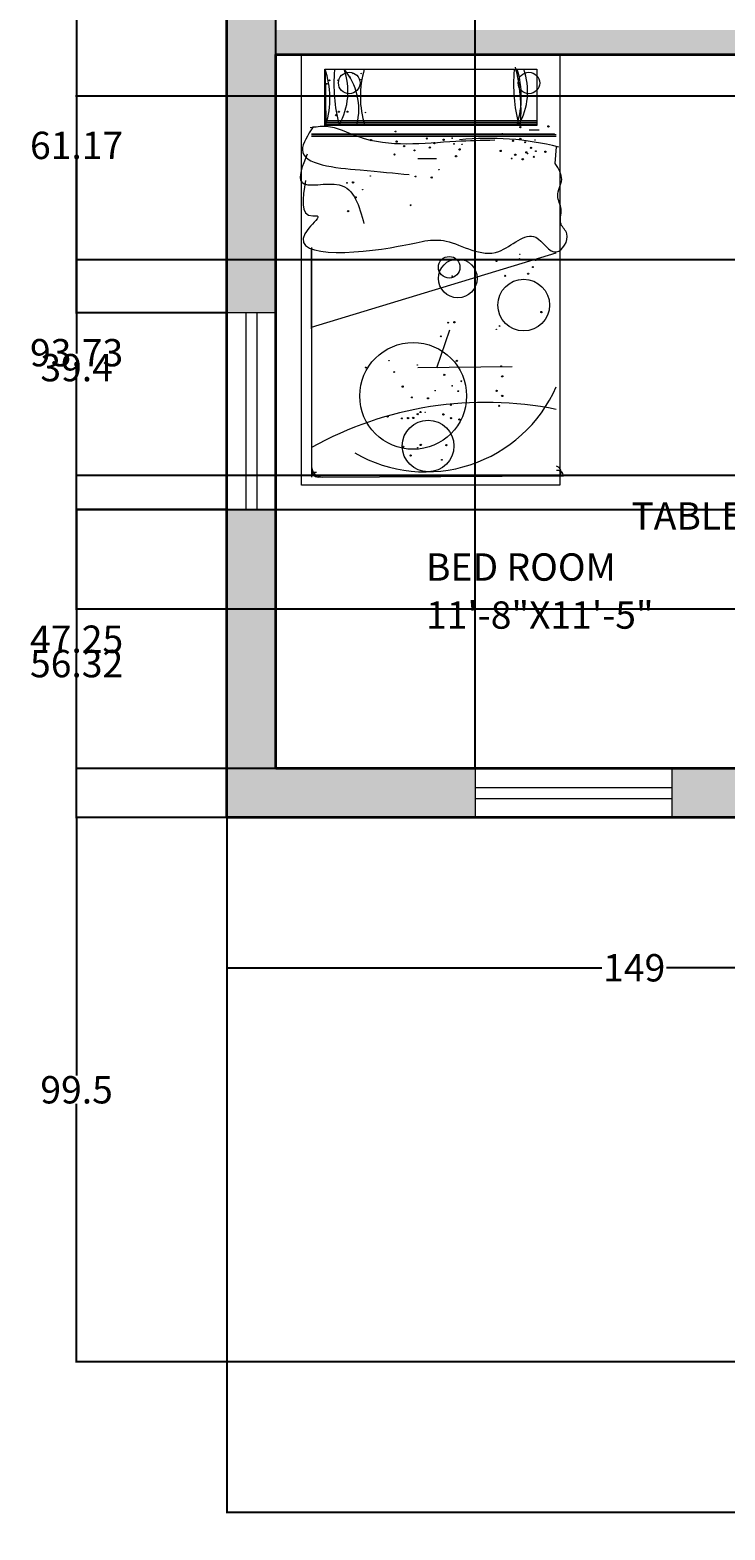
# Model space of a CAD drawing. Units: inches. Extents: x 2807 to 3326, y 2005 to 2580.
# Tile 1 of 12: x 2809 to 2936, y 2005 to 2280. Entities that reach past the tile are written whole.
import ezdxf

# ---------------------------------------------------------------- set-up
doc = ezdxf.new("R2010")
doc.units = ezdxf.units.IN
doc.header["$LTSCALE"] = 0.4
for name, color, linetype, lineweight in [('A-ANNO-DIMS', 2, 'Continuous', 18), ('A-AREA-IDEN', 5, 'Continuous', 18), ('A-WALL-PATT', 231, 'Continuous', 13), ('Furniture', 7, 'Continuous', 15), ('WALL', 233, 'Continuous', 35), ('WINDOWS', 132, 'Continuous', 18)]:
    doc.layers.add(name, color=color, linetype=linetype, lineweight=lineweight)
doc.styles.get("Standard").update_dxf_attribs({"font": 'txt', "height": 5})
doc.dimstyles.get("Standard").update_dxf_attribs({"dimtxt": 0.18, "dimasz": 0.18, "dimexe": 0.18, "dimexo": 0.0625, "dimgap": 0.09, "dimtad": 0, "dimtih": 1, "dimtoh": 1, "dimdec": 4, "dimzin": 0, "dimdsep": 46, "dimtxsty": 'Standard', "dimcen": 0.09, "dimadec": 0, "dimazin": 0, "dimtfac": 1, "dimtdec": 4, "dimtofl": 0, "dimtmove": 0, "dimatfit": 3, "dimfxl": 1, "dimtolj": 1, "dimtzin": 0, "dimarcsym": 0})

# ---------------------------------------------------------------- blocks, each defined once
blk = doc.blocks.new('WIN-36')
at = {"ltscale": 0.4}
for p, q in [((0, 36), (0, 0)), ((9, 36), (0, 36)), ((3.5, 36), (3.5, 0)), ((5.5, 36), (5.5, 0)), ((9, 0), (9, 36)), ((0, 0), (9, 0))]:
    blk.add_line(p, q, dxfattribs=at)
blk = doc.blocks.new('BED-SINGLE')
for p, q in [((-24.2, -78.74), (-24.2, 0)), ((23.05, 0), (-24.2, 0)), ((23.05, 0), (23.05, -78.74)), ((-19.91, -2.64), (18.85, -2.64)), ((-19.91, -12.97), (-19.91, -2.64)), ((-19.86, -2.65), (-19.71, -12.79)), ((18.85, -2.64), (18.85, -12.97)), ((18.85, -12.97), (-19.91, -12.97)), ((-19.71, -12.07), (18.88, -12.07)), ((-19.71, -12.36), (18.88, -12.36)), ((-19.71, -12.66), (18.88, -12.66)), ((-19.71, -12.79), (18.88, -12.79)), ((-22.36, -14.62), (22.4, -14.6)), ((-22.36, -14.92), (22.4, -14.9)), ((-22.34, -14.47), (22.1, -14.45)), ((19.29, -13.84), (17.45, -13.84)), ((0.5, -19.06), (-2.92, -19.06)), ((22.21, -19.89), (22.42, -16.84)), ((-22.34, -35.25), (-22.34, -77.26)), ((-22.34, -35.25), (-22.34, -75.28)), ((-22.34, -50.11), (-22.34, -35.53)), ((-22.36, -49.81), (22.4, -36.21)), ((2.87, -50.36), (0.49, -57.3)), ((14.32, -57.07), (-2.92, -57.29)), ((-22.21, -76.32), (-21.42, -76.32)), ((23.05, -78.74), (-24.2, -78.74)), ((-21.16, -77.25), (23.72, -77.02))]:
    blk.add_line(p, q)
for centre, radius in [((-19.54, -5.33), 0.0787), ((-19.07, -4.7), 0.0787), ((-17.49, -4.7), 0.0787), ((-15.45, -5.18), 1.97), ((-15.29, -4.08), 0.0394), ((-14.82, -3.45), 0.0394), ((-13.24, -3.45), 0.0394), ((-13.24, -4.55), 0.0394), ((17.4, -5.19), 1.97), ((-17.82, -11.05), 0.118), ((-17.35, -10.43), 0.118), ((-15.77, -10.43), 0.118), ((-12.46, -10.58), 0.0394), ((15.84, -13.26), 0.118), ((20.96, -13.12), 0.118), ((-11.46, -15.62), 0.118), ((-6.97, -14.05), 0.0787), ((-6.78, -15.9), 0.118), ((-1.26, -15.34), 0.118), ((0.11, -16.17), 0.118), ((1.8, -15.56), 0.118), ((3.7, -16.3), 0.0787), ((5.19, -16.39), 0.0394), ((12.55, -14.52), 0.118), ((14.47, -15.76), 0.118), ((15.82, -15.39), 0.118), ((16.73, -16.02), 0.0787), ((17.27, -14.65), 0.0394), ((18.52, -15.61), 0.0394), ((-7.18, -18.26), 0.118), ((-5.4, -16.72), 0.118), ((-3.52, -17.51), 0.0787), ((-0.71, -17), 0.118), ((4.08, -18.58), 0.118), ((4.72, -17.32), 0.118), ((12.24, -17.6), 0.118), ((14.25, -19), 0.0787), ((14.9, -18.3), 0.118), ((16.28, -19.13), 0.118), ((16.93, -17.87), 0.118), ((17.15, -18.11), 0.0394), ((17.76, -17.04), 0.118), ((18.3, -18.69), 0.118), ((18.66, -17.64), 0.0787), ((20.41, -17.75), 0.118), ((0.94, -21.04), 0.0394), ((-15.86, -23.43), 0.0787), ((-14.74, -23.37), 0.118), ((-12.98, -24.68), 0.0394), ((-11.61, -22.18), 0.0394), ((-3.31, -22.29), 0.0787), ((-0.37, -22.46), 0.118), ((-14.28, -26.11), 0.118), ((-15.65, -28.61), 0.118), ((-4.22, -27.54), 0.0787), ((2.83, -38.87), 1.97), ((4.4, -40.91), 3.54), ((4.64, -37.58), 0.0394), ((11.49, -37.77), 0.0787), ((15.68, -37.38), 0.0787), ((15.74, -36.51), 0.0394), ((18.63, -37.54), 0.118), ((16.45, -45.79), 4.72), ((13.06, -40.44), 0.118), ((17.26, -40.05), 0.118), ((18.11, -38.84), 0.0787), ((2.65, -49), 0.0787), ((3.77, -48.94), 0.118), ((19.68, -47.06), 0.118), ((1.28, -51.5), 0.0787), ((11.44, -50.24), 0.0394), ((12.05, -49.61), 0.0787), ((-3.76, -62.4), 9.76), ((-12.43, -57.2), 0.0787), ((-8.18, -55.94), 0.0394), ((-3, -56.76), 0.0394), ((4.23, -56), 0.118), ((12.32, -56.97), 0.0787), ((-7.25, -58.02), 0.0787), ((1.92, -58.54), 0.118), ((5.04, -59.72), 0.0787), ((12.52, -58.82), 0.118), ((-5.68, -60.69), 0.118), ((-3.99, -62.67), 0.0787), ((-1.05, -62.84), 0.118), ((0.26, -61.41), 0.0394), ((4.48, -61.53), 0.0787), ((11.5, -61.47), 0.118), ((12.52, -62.39), 0.118), ((-2.92, -65.73), 0.118), ((-2.42, -65.34), 0.118), ((-1.57, -65.38), 0.0394), ((1.77, -65.78), 0.118), ((3.11, -64.04), 0.0787), ((11.96, -64.21), 0.118), ((-8.43, -66.14), 0.118), ((-5.82, -66.51), 0.0787), ((-1.03, -71.55), 4.72), ((-4.7, -66.45), 0.118), ((-3.75, -66.42), 0.118), ((3.15, -66.47), 0.118), ((4.68, -66.71), 0.118), ((-2.37, -71.35), 0.118), ((2.32, -71.4), 0.118), ((-5.61, -71.69), 0.118), ((-4.24, -73.29), 0.118), ((-2.94, -71.86), 0.0394), ((1.48, -74.08), 0.0787)]:
    blk.add_circle(centre, radius)
for centre, radius, start, end in [((-35.51, -7.95), 16.53, 343.0006, 18.6759), ((-27.69, -6.75), 12.01, 329.8072, 19.9256), ((-25.06, -10.01), 11.36, 345.8396, 40.337), ((4.43, -7.67), 17.85, 163.6634, 197.1743), ((-14.89, -10.2), 30.85, 355.6161, 14.8863), ((-1.49, -7.71), 17.5, 343.1329, 16.7593), ((5.16, -6.76), 12.01, 329.8072, 19.9256), ((10.58, -5.48), 28.83, 174.7074, 194.6885), ((43.43, -5.5), 28.83, 174.7074, 194.6885), ((10.02, -67.77), 52.46, 75.8437, 95.7821), ((-1.46, -50.2), 26.08, 240.1506, 336.1931), ((9.49, -129.11), 65.53, 78.633, 119.0775), ((-20.37, -75.28), 1.97, 180, 270), ((-21.16, -76.07), 1.18, 180, 270), ((22.26, -76.26), 1.02, 311.9337, 80.5378), ((22.61, -77.16), 1.13, 7.0311, 99.2977)]:
    blk.add_arc(centre, radius, start, end)
for points, knots in [([(-22, -13.16), (-23.02, -14.71), (-26.47, -19.94), (-13.14, -21.11), (-7.15, -21.67), (-4.47, -21.92)], [0, 0, 0, 0, 4.712342, 15.867179, 24.91455, 24.91455, 24.91455, 24.91455]), ([(11.17, -15.66), (8.81, -15.7), (0.54, -15.87), (-10.21, -17.37), (-18.53, -12.79), (-21.61, -13.25), (-22.61, -13.4)], [0, 0, 0, 0, 7.121262, 24.909491, 31.123221, 34.101394, 34.101394, 34.101394, 34.101394]), ([(-23.16, -18.18), (-24, -20.34), (-25.96, -25.33), (-15.15, -21.84), (-13.61, -27.69), (-12.77, -30.9)], [0, 0, 0, 0, 5.247261, 12.129135, 20.530793, 20.530793, 20.530793, 20.530793]), ([(-23.42, -23.01), (-23.98, -26.23), (-24.61, -29.87), (-20.32, -29.28), (-30.03, -37.77), (-6.68, -35.83), (2.09, -32.61), (11.16, -38.92), (18.11, -30.55), (22.1, -38.17), (25.33, -33.01), (22.67, -30.96), (23.73, -28.27), (22.1, -25.67), (24.04, -22.75), (22.83, -20.86), (22.21, -19.89)], [0, 0, 0, 0, 6.608381, 7.436978, 10.160479, 26.82811, 35.651646, 45.441607, 52.697614, 57.347481, 61.162366, 63.231685, 65.951856, 68.505046, 71.545852, 74.730692, 74.730692, 74.730692, 74.730692])]:
    blk.add_open_spline(points, degree=3, knots=knots)
for p in [(3.38, -15.28), (3.38, -40.49), (3.38, -60.57)]:
    blk.add_point(p)
blk = doc.blocks.new('*D29')
at = {"layer": 'A-ANNO-DIMS', "color": 0, "lineweight": -2, "ltscale": 0.4, "transparency": 16777216}
for p, q in [((2959.79, 2230.64), (2947.71, 2230.64)), ((2947.89, 2230.46), (2947.89, 2193.32)), ((2947.89, 2151.01), (2947.89, 2188.14)), ((2959.79, 2150.83), (2947.71, 2150.83))]:
    blk.add_line(p, q, dxfattribs=at)
at = {"layer": 'A-ANNO-DIMS', "color": 0, "ltscale": 0.4, "transparency": 16777216}
for points in [[(2947.86, 2230.46), (2947.92, 2230.46), (2947.89, 2230.64)], [(2947.86, 2151.01), (2947.92, 2151.01), (2947.89, 2150.83)]]:
    blk.add_solid(points, dxfattribs=at)
at = {"layer": 'Defpoints', "color": 0, "ltscale": 0.4, "transparency": 16777216}
for p in [(2947.89, 2230.64), (2959.86, 2230.64), (2959.86, 2150.83)]:
    blk.add_point(p, dxfattribs=at)
at = {"layer": 'A-ANNO-DIMS', "color": 0, "ltscale": 0.4, "transparency": 16777216, "insert": (2947.89, 2190.73), "char_height": 5, "attachment_point": 5}
blk.add_mtext('\\A1;TABLE SET 80 TYP.', dxfattribs=at)
blk = doc.blocks.new('*D31')
at = {"layer": 'A-ANNO-DIMS', "color": 0, "lineweight": -2, "ltscale": 0.4, "transparency": 16777216}
for p, q in [((2844.57, 2135.51), (2844.57, 2008.45)), ((3288.57, 2135.51), (3288.57, 2008.45)), ((2844.75, 2008.63), (3059.93, 2008.63)), ((3288.39, 2008.63), (3073.2, 2008.63))]:
    blk.add_line(p, q, dxfattribs=at)
at = {"layer": 'A-ANNO-DIMS', "color": 0, "ltscale": 0.4, "transparency": 16777216}
for points in [[(2844.75, 2008.66), (2844.75, 2008.6), (2844.57, 2008.63)], [(3288.39, 2008.66), (3288.39, 2008.6), (3288.57, 2008.63)]]:
    blk.add_solid(points, dxfattribs=at)
at = {"layer": 'Defpoints', "color": 0, "ltscale": 0.4, "transparency": 16777216}
for p in [(2844.57, 2135.58), (3288.57, 2135.58), (3288.57, 2008.63)]:
    blk.add_point(p, dxfattribs=at)
at = {"layer": 'A-ANNO-DIMS', "color": 0, "ltscale": 0.4, "transparency": 16777216, "insert": (3066.57, 2008.63), "char_height": 5, "attachment_point": 5}
blk.add_mtext('\\A1;444', dxfattribs=at)
blk = doc.blocks.new('*D33')
at = {"layer": 'A-ANNO-DIMS', "color": 0, "lineweight": -2, "ltscale": 0.4, "transparency": 16777216}
for p, q in [((2844.504691, 2135.576496), (2816.937191, 2135.576496)), ((2817.117191, 2135.396496), (2817.117191, 2088.416496)), ((2817.117191, 2036.256496), (2817.117191, 2083.236496)), ((2984.504691, 2036.076496), (2816.937191, 2036.076496))]:
    blk.add_line(p, q, dxfattribs=at)
at = {"layer": 'A-ANNO-DIMS', "color": 0, "ltscale": 0.4, "transparency": 16777216}
for points in [[(2817.087191, 2135.396496), (2817.147191, 2135.396496), (2817.117191, 2135.576496)], [(2817.087191, 2036.256496), (2817.147191, 2036.256496), (2817.117191, 2036.076496)]]:
    blk.add_solid(points, dxfattribs=at)
at = {"layer": 'Defpoints', "color": 0, "ltscale": 0.4, "transparency": 16777216}
for p in [(2817.117191, 2135.576496), (2844.567191, 2135.576496), (2984.567191, 2036.076496)]:
    blk.add_point(p, dxfattribs=at)
at = {"layer": 'A-ANNO-DIMS', "color": 0, "ltscale": 0.4, "transparency": 16777216, "insert": (2817.117191, 2085.826496), "char_height": 5, "attachment_point": 5}
blk.add_mtext('\\A1;99.5', dxfattribs=at)
blk = doc.blocks.new('*D35')
at = {"layer": 'A-ANNO-DIMS', "color": 0, "lineweight": -2, "ltscale": 0.4, "transparency": 16777216}
for p, q in [((2844.57, 2135.51), (2844.57, 2107.95)), ((2993.57, 2135.51), (2993.57, 2107.95)), ((2844.75, 2108.13), (2913.14, 2108.13)), ((2993.39, 2108.13), (2924.99, 2108.13))]:
    blk.add_line(p, q, dxfattribs=at)
at = {"layer": 'A-ANNO-DIMS', "color": 0, "ltscale": 0.4, "transparency": 16777216}
for points in [[(2844.75, 2108.16), (2844.75, 2108.1), (2844.57, 2108.13)], [(2993.39, 2108.16), (2993.39, 2108.1), (2993.57, 2108.13)]]:
    blk.add_solid(points, dxfattribs=at)
at = {"layer": 'Defpoints', "color": 0, "ltscale": 0.4, "transparency": 16777216}
for p in [(2844.57, 2135.58), (2993.57, 2135.58), (2844.57, 2108.13)]:
    blk.add_point(p, dxfattribs=at)
at = {"layer": 'A-ANNO-DIMS', "color": 0, "ltscale": 0.4, "transparency": 16777216, "insert": (2919.07, 2108.13), "char_height": 5, "attachment_point": 5}
blk.add_mtext('\\A1;149', dxfattribs=at)
blk = doc.blocks.new('*D37')
at = {"layer": 'A-ANNO-DIMS', "color": 0, "lineweight": -2, "ltscale": 0.4, "transparency": 16777216}
for p, q in [((2853.567191, 2144.638996), (2853.567191, 2577.206496)), ((2853.747191, 2577.026496), (2859.189306, 2577.026496)), ((2889.811421, 2577.026496), (2884.369306, 2577.026496)), ((2889.991421, 2144.638996), (2889.991421, 2577.206496))]:
    blk.add_line(p, q, dxfattribs=at)
at = {"layer": 'A-ANNO-DIMS', "color": 0, "ltscale": 0.4, "transparency": 16777216}
for points in [[(2853.747191, 2577.056496), (2853.747191, 2576.996496), (2853.567191, 2577.026496)], [(2889.811421, 2577.056496), (2889.811421, 2576.996496), (2889.991421, 2577.026496)]]:
    blk.add_solid(points, dxfattribs=at)
at = {"layer": 'Defpoints', "color": 0, "ltscale": 0.4, "transparency": 16777216}
for p in [(2889.991421, 2577.026496), (2853.567191, 2144.576496), (2889.991421, 2144.576496)]:
    blk.add_point(p, dxfattribs=at)
at = {"layer": 'A-ANNO-DIMS', "color": 0, "ltscale": 0.4, "transparency": 16777216, "insert": (2871.779306, 2577.026496), "char_height": 5, "attachment_point": 5}
blk.add_mtext('\\A1;36.424', dxfattribs=at)
blk = doc.blocks.new('*D41')
at = {"layer": 'A-ANNO-DIMS', "color": 0, "lineweight": -2, "ltscale": 0.4, "transparency": 16777216}
for p, q in [((2844.5, 2191.9), (2816.94, 2191.9)), ((2817.12, 2191.72), (2817.12, 2166.33)), ((2817.12, 2135.76), (2817.12, 2161.15)), ((2844.5, 2135.58), (2816.94, 2135.58))]:
    blk.add_line(p, q, dxfattribs=at)
at = {"layer": 'A-ANNO-DIMS', "color": 0, "ltscale": 0.4, "transparency": 16777216}
for points in [[(2817.09, 2191.72), (2817.15, 2191.72), (2817.12, 2191.9)], [(2817.09, 2135.76), (2817.15, 2135.76), (2817.12, 2135.58)]]:
    blk.add_solid(points, dxfattribs=at)
at = {"layer": 'Defpoints', "color": 0, "ltscale": 0.4, "transparency": 16777216}
for p in [(2817.12, 2191.9), (2844.57, 2191.9), (2844.57, 2135.58)]:
    blk.add_point(p, dxfattribs=at)
at = {"layer": 'A-ANNO-DIMS', "color": 0, "ltscale": 0.4, "transparency": 16777216, "insert": (2817.12, 2163.74), "char_height": 5, "attachment_point": 5}
blk.add_mtext('\\A1;56.32', dxfattribs=at)
blk = doc.blocks.new('*D42')
at = {"layer": 'A-ANNO-DIMS', "color": 0, "lineweight": -2, "ltscale": 0.4, "transparency": 16777216}
for p, q in [((2844.504691, 2289.066335), (2816.937191, 2289.066335)), ((2817.117191, 2288.886335), (2817.117191, 2261.071202)), ((2817.117191, 2228.076069), (2817.117191, 2255.891202)), ((2844.504691, 2227.896069), (2816.937191, 2227.896069))]:
    blk.add_line(p, q, dxfattribs=at)
at = {"layer": 'A-ANNO-DIMS', "color": 0, "ltscale": 0.4, "transparency": 16777216}
for points in [[(2817.087191, 2288.886335), (2817.147191, 2288.886335), (2817.117191, 2289.066335)], [(2817.087191, 2228.076069), (2817.147191, 2228.076069), (2817.117191, 2227.896069)]]:
    blk.add_solid(points, dxfattribs=at)
at = {"layer": 'Defpoints', "color": 0, "ltscale": 0.4, "transparency": 16777216}
for p in [(2817.117191, 2289.066335), (2844.567191, 2289.066335), (2844.567191, 2227.896069)]:
    blk.add_point(p, dxfattribs=at)
at = {"layer": 'A-ANNO-DIMS', "color": 0, "ltscale": 0.4, "transparency": 16777216, "insert": (2817.117191, 2258.481202), "char_height": 5, "attachment_point": 5}
blk.add_mtext('\\A1;61.17', dxfattribs=at)
blk = doc.blocks.new('*D45')
at = {"layer": 'A-ANNO-DIMS', "color": 0, "lineweight": -2, "ltscale": 0.4, "transparency": 16777216}
for p, q in [((3279.504691, 2191.826496), (2816.937191, 2191.826496)), ((2817.117191, 2191.646496), (2817.117191, 2170.791496)), ((2817.117191, 2144.756496), (2817.117191, 2165.611496)), ((3279.504691, 2144.576496), (2816.937191, 2144.576496))]:
    blk.add_line(p, q, dxfattribs=at)
at = {"layer": 'A-ANNO-DIMS', "color": 0, "ltscale": 0.4, "transparency": 16777216}
for points in [[(2817.087191, 2191.646496), (2817.147191, 2191.646496), (2817.117191, 2191.826496)], [(2817.087191, 2144.756496), (2817.147191, 2144.756496), (2817.117191, 2144.576496)]]:
    blk.add_solid(points, dxfattribs=at)
at = {"layer": 'Defpoints', "color": 0, "ltscale": 0.4, "transparency": 16777216}
for p in [(2817.117191, 2191.826496), (3279.567191, 2191.826496), (3279.567191, 2144.576496)]:
    blk.add_point(p, dxfattribs=at)
at = {"layer": 'A-ANNO-DIMS', "color": 0, "ltscale": 0.4, "transparency": 16777216, "insert": (2817.117191, 2168.201496), "char_height": 5, "attachment_point": 5}
blk.add_mtext('\\A1;47.25', dxfattribs=at)
blk = doc.blocks.new('*D61')
at = {"layer": 'A-ANNO-DIMS', "color": 0, "lineweight": -2, "ltscale": 0.4, "transparency": 16777216}
for p, q in [((3088.922898, 2267.452063), (2816.937191, 2267.452063)), ((2817.117191, 2267.272063), (2817.117191, 2223.175564)), ((2817.117191, 2173.899065), (2817.117191, 2217.995564)), ((3079.479513, 2173.719065), (2816.937191, 2173.719065))]:
    blk.add_line(p, q, dxfattribs=at)
at = {"layer": 'A-ANNO-DIMS', "color": 0, "ltscale": 0.4, "transparency": 16777216}
for points in [[(2817.087191, 2267.272063), (2817.147191, 2267.272063), (2817.117191, 2267.452063)], [(2817.087191, 2173.899065), (2817.147191, 2173.899065), (2817.117191, 2173.719065)]]:
    blk.add_solid(points, dxfattribs=at)
at = {"layer": 'Defpoints', "color": 0, "ltscale": 0.4, "transparency": 16777216}
for p in [(2817.117191, 2267.452063), (3088.985398, 2267.452063), (3079.542013, 2173.719065)]:
    blk.add_point(p, dxfattribs=at)
at = {"layer": 'A-ANNO-DIMS', "color": 0, "ltscale": 0.4, "transparency": 16777216, "insert": (2817.117191, 2220.585564), "char_height": 5, "attachment_point": 5}
blk.add_mtext('\\A1;93.73', dxfattribs=at)
blk = doc.blocks.new('*D65')
at = {"layer": 'A-ANNO-DIMS', "color": 0, "lineweight": -2, "ltscale": 0.4, "transparency": 16777216}
for p, q in [((3080.36, 2237.55), (2816.94, 2237.55)), ((2817.12, 2237.37), (2817.12, 2220.44)), ((2817.12, 2198.33), (2817.12, 2215.26)), ((3080.36, 2198.15), (2816.94, 2198.15))]:
    blk.add_line(p, q, dxfattribs=at)
at = {"layer": 'A-ANNO-DIMS', "color": 0, "ltscale": 0.4, "transparency": 16777216}
for points in [[(2817.09, 2237.37), (2817.15, 2237.37), (2817.12, 2237.55)], [(2817.09, 2198.33), (2817.15, 2198.33), (2817.12, 2198.15)]]:
    blk.add_solid(points, dxfattribs=at)
at = {"layer": 'Defpoints', "color": 0, "ltscale": 0.4, "transparency": 16777216}
for p in [(2817.12, 2237.55), (3080.43, 2237.55), (3080.43, 2198.15)]:
    blk.add_point(p, dxfattribs=at)
at = {"layer": 'A-ANNO-DIMS', "color": 0, "ltscale": 0.4, "transparency": 16777216, "insert": (2817.12, 2217.85), "char_height": 5, "attachment_point": 5}
blk.add_mtext('\\A1;39.4', dxfattribs=at)

msp = doc.modelspace()

# ---------------------------------------------------------------- hatches: boundary and pattern name
at = {"layer": 'A-WALL-PATT', "ltscale": 0.4}
h = msp.add_hatch(color=256, dxfattribs=at)
h.dxf.hatch_style = 1
h.paths.add_polyline_path([(3288.5672, 2549.5765), (2941.5672, 2549.5765), (2941.5672, 2540.5765), (2993.5672, 2540.5765), (2993.5672, 2489.5693), (2998.0672, 2489.5693), (2998.0672, 2540.5765), (3135.0672, 2540.5765), (3135.0672, 2479.0765), (3139.5672, 2479.0765), (3139.5672, 2540.5765), (3279.5672, 2540.5765), (3279.5672, 2510.5765), (3288.5672, 2510.5765)])
h.paths.add_polyline_path([(2905.5672, 2549.5765), (2844.5672, 2549.5765), (2844.5672, 2445.94), (2853.5672, 2445.94), (2853.5672, 2540.5765), (2905.5672, 2540.5765)])
h.paths.add_polyline_path([(2853.5672, 2409.94), (2844.5672, 2409.94), (2844.5672, 2371.3497), (2853.5672, 2371.3497), (2853.5672, 2380.0765), (2909.0672, 2380.0765), (2909.0672, 2384.5765), (2853.5672, 2384.5765)])
h.paths.add_polyline_path([(2998.0672, 2389.0765), (2993.5672, 2389.0765), (2993.5672, 2384.5765), (2939.0672, 2384.5765), (2939.0672, 2380.0765), (2943.5672, 2380.0765), (2943.5672, 2314.0765), (2948.0672, 2314.0765), (2948.0672, 2380.0765), (2998.0672, 2380.0765)])
h.paths.add_polyline_path([(2998.0672, 2471.8029), (2993.5672, 2471.8029), (2993.5672, 2425.0765), (2998.0672, 2425.0765)])
h.paths.add_polyline_path([(2953.0672, 2279.5765), (2948.0672, 2279.5765), (2948.0672, 2284.0765), (2943.5672, 2284.0765), (2943.5672, 2279.5765), (2853.5672, 2279.5765), (2853.5672, 2289.0663), (2844.5672, 2289.0663), (2844.5672, 2227.8961), (2853.5672, 2227.8961), (2853.5672, 2275.0765), (2953.0672, 2275.0765)])
h.paths.add_polyline_path([(2943.5672, 2332.0765), (2853.5672, 2332.0765), (2853.5672, 2347.3497), (2844.5672, 2347.3497), (2844.5672, 2313.0663), (2853.5672, 2313.0663), (2853.5672, 2327.5765), (2943.5672, 2327.5765)])
h.paths.add_polyline_path([(3144.0672, 2279.5765), (2993.5672, 2279.5765), (2989.0672, 2279.5765), (2989.0672, 2275.0765), (2993.5672, 2275.0765), (2993.5672, 2144.5765), (2984.5672, 2144.5765), (2984.5672, 2135.5765), (2993.5672, 2135.5765), (2993.5672, 2120.0765), (3036.5672, 2120.0765), (3036.5672, 2129.0765), (2998.0672, 2129.0765), (2998.0672, 2275.0765), (3135.0672, 2275.0765), (3135.0672, 2129.0765), (3096.5672, 2129.0765), (3096.5672, 2120.0765), (3139.5672, 2120.0765), (3139.5672, 2135.5765), (3148.5672, 2135.5765), (3148.5672, 2144.5765), (3139.5672, 2144.5765), (3139.5672, 2275.0765), (3144.0672, 2275.0765)])
h.paths.add_polyline_path([(2984.5672, 2144.5765), (2925.9914, 2144.5765), (2925.9914, 2135.5765), (2984.5672, 2135.5765)])
h.paths.add_polyline_path([(2889.9914, 2144.5765), (2853.5672, 2144.5765), (2853.5672, 2191.8961), (2844.5672, 2191.8961), (2844.5672, 2135.5765), (2889.9914, 2135.5765)])
h.paths.add_polyline_path([(3196.0672, 2144.5765), (3148.5672, 2144.5765), (3148.5672, 2135.5765), (3196.0672, 2135.5765)])
h.paths.add_polyline_path([(3288.5672, 2191.8265), (3279.5672, 2191.8265), (3279.5672, 2144.5765), (3232.0672, 2144.5765), (3232.0672, 2135.5765), (3288.5672, 2135.5765)])
h.paths.add_polyline_path([(3288.5672, 2292.8229), (3279.5672, 2292.8229), (3279.5672, 2291.4371), (3279.5672, 2279.5765), (3189.5672, 2279.5765), (3189.5672, 2293.0765), (3185.0672, 2293.0765), (3185.0672, 2279.5765), (3180.0672, 2279.5765), (3180.0672, 2275.0765), (3279.5672, 2275.0765), (3279.5672, 2227.8265), (3288.5672, 2227.8265)])
h.paths.add_polyline_path([(3288.5672, 2368.0765), (3279.5672, 2368.0765), (3279.5672, 2332.0765), (3174.0672, 2332.0765), (3174.0672, 2327.5765), (3185.0672, 2327.5765), (3189.5672, 2327.5765), (3279.5672, 2327.5765), (3279.5672, 2316.8229), (3288.5672, 2316.8229)])
h.paths.add_polyline_path([(3288.5672, 2474.5765), (3279.5672, 2474.5765), (3279.5672, 2444.5765), (3139.5672, 2444.5765), (3139.5672, 2449.0765), (3135.0672, 2449.0765), (3135.0672, 2327.5765), (3144.0672, 2327.5765), (3144.0672, 2332.0765), (3139.5672, 2332.0765), (3139.5672, 2440.0765), (3279.5672, 2440.0765), (3279.5672, 2404.0765), (3288.5672, 2404.0765)])

# ---------------------------------------------------------------- linework, layer by layer
at = {"layer": 'WALL'}
for p, q in [((2844.5672, 2135.5765), (2844.5672, 2549.5765)), ((2853.5672, 2144.5765), (2853.5672, 2275.0765)), ((2853.5672, 2275.0765), (2953.0672, 2275.0765)), ((2993.5672, 2144.5765), (2853.5672, 2144.5765)), ((2993.5672, 2135.5765), (2844.5672, 2135.5765))]:
    msp.add_line(p, q, dxfattribs=at)

# ---------------------------------------------------------------- block references
at = {"layer": 'Furniture'}
msp.add_blockref('BED-SINGLE', (2882.415, 2275.076), dxfattribs=at)
at = {"layer": 'WINDOWS'}
msp.add_blockref('WIN-36', (2844.5672, 2191.8961), dxfattribs=at)
at = {"layer": 'WINDOWS', "rotation": 89.99999999999696}
msp.add_blockref('WIN-36', (2925.9914, 2135.5765), dxfattribs=at)

# ---------------------------------------------------------------- texts
at = {"layer": 'A-AREA-IDEN', "ltscale": 0.4}
for s, p in [('BED ROOM', (2880.9986, 2178.8956)), ('11\'-8"X11\'-5"', (2880.9986, 2170.1217))]:
    msp.add_text(s, height=5, dxfattribs=at).set_placement(p)

# ---------------------------------------------------------------- dimensions: what is measured, and where the dimension line sits
at = {"layer": 'A-ANNO-DIMS', "ltscale": 0.4}
for base, p1, p2, override, picture, middle in [((2889.9914, 2577.0265), (2853.5672, 2144.5765), (2889.9914, 2144.5765), {"dimdec": 3, "dimlfac": 1, "dimrnd": 0, "dimzin": 0, "dimdsep": 46, "dimlunit": 2}, '*D37', (2871.7793, 2577.0265)), ((3288.5672, 2008.6265), (2844.5672, 2135.5765), (3288.5672, 2135.5765), {"dimdec": 0, "dimlfac": 1, "dimrnd": 0, "dimzin": 0, "dimdsep": 46, "dimlunit": 2}, '*D31', (3066.5672, 2008.6265))]:
    dim = msp.add_linear_dim(base=base, p1=p1, p2=p2, dimstyle='Standard', override=override, dxfattribs=at)
    dim.commit()
    dim.dimension.update_dxf_attribs({"geometry": picture, "text_midpoint": middle})
for base, p1, p2, angle, override, picture, middle in [((2817.1172, 2289.0663), (2844.5672, 2227.8961), (2844.5672, 2289.0663), 90, {"dimdec": 2, "dimlfac": 1, "dimrnd": 0, "dimzin": 0, "dimdsep": 46, "dimlunit": 2}, '*D42', (2817.1172, 2258.4812)), ((2817.1172, 2267.4521), (3079.542, 2173.7191), (3088.9854, 2267.4521), 90, {"dimdec": 2, "dimlfac": 1, "dimrnd": 0, "dimzin": 0, "dimdsep": 46, "dimlunit": 2}, '*D61', (2817.1172, 2220.5856)), ((2817.1172, 2237.5518), (3080.4262, 2198.1526), (3080.4262, 2237.5518), 90, {"dimdec": 1, "dimlfac": 1, "dimrnd": 0, "dimzin": 0, "dimdsep": 46, "dimlunit": 2}, '*D65', (2817.1172, 2217.8522)), ((2817.1172, 2191.8961), (2844.5672, 2135.5765), (2844.5672, 2191.8961), 90, {"dimdec": 2, "dimlfac": 1, "dimrnd": 0, "dimzin": 0, "dimdsep": 46, "dimlunit": 2}, '*D41', (2817.1172, 2163.7363)), ((2817.1172, 2191.8265), (3279.5672, 2144.5765), (3279.5672, 2191.8265), 90, {"dimdec": 2, "dimlfac": 1, "dimrnd": 0, "dimzin": 0, "dimdsep": 46, "dimlunit": 2}, '*D45', (2817.1172, 2168.2015)), ((2817.1172, 2135.5765), (2984.5672, 2036.0765), (2844.5672, 2135.5765), 90, {"dimdec": 1, "dimlfac": 1, "dimrnd": 0, "dimzin": 0, "dimdsep": 46, "dimlunit": 2}, '*D33', (2817.1172, 2085.8265)), ((2844.5672, 2108.1265), (2993.5672, 2135.5765), (2844.5672, 2135.5765), 180, {"dimdec": 0, "dimlfac": 1, "dimrnd": 0, "dimzin": 0, "dimdsep": 46, "dimlunit": 2}, '*D35', (2919.0672, 2108.1265))]:
    dim = msp.add_linear_dim(base=base, p1=p1, p2=p2, angle=angle, dimstyle='Standard', override=override, dxfattribs=at)
    dim.commit()
    dim.dimension.update_dxf_attribs({"geometry": picture, "text_midpoint": middle})
dim = msp.add_linear_dim(base=(2947.8868, 2230.6362), p1=(2959.8575, 2150.8316), p2=(2959.8575, 2230.6362), angle=90, text='TABLE SET <> TYP.', dimstyle='Standard', override={"dimdec": 0, "dimlfac": 1, "dimrnd": 0, "dimzin": 0, "dimdsep": 46, "dimlunit": 2}, dxfattribs=at)
dim.commit()
dim.dimension.update_dxf_attribs({"geometry": '*D29', "text_midpoint": (2947.8868, 2190.7339)})

doc.saveas('drawing.dxf')
